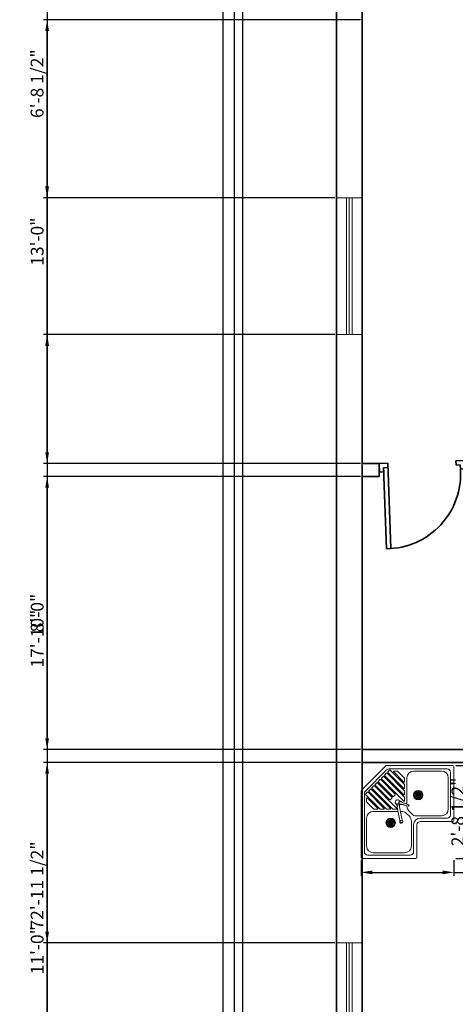
# Model space of a CAD drawing. Units: inches. Extents: x 1239 to 2276906, y 2273 to 321338.
# Tile 15 of 23: x 1239 to 1392, y 3026 to 3372. Entities that reach past the tile are written whole.
import ezdxf

# ---------------------------------------------------------------- set-up
doc = ezdxf.new("R2010")
doc.units = ezdxf.units.IN
for name, color, linetype, lineweight in [('A-ANNO-DIMS', 2, 'Continuous', 18), ('A-FLOR-FIXT', 9, 'Continuous', 18), ('C-PROP', 7, 'Continuous', 25), ('DOOR', 1, 'Continuous', 25), ('wall', 7, 'Continuous', 35), ('WINDOW', 50, 'Continuous', 18)]:
    doc.layers.add(name, color=color, linetype=linetype, lineweight=lineweight)
doc.styles.get("Standard").update_dxf_attribs({"font": 'arial.ttf'})
doc.dimstyles.new('ISO-25', dxfattribs={"dimtxt": 4.5, "dimasz": 4, "dimexe": 1.25, "dimexo": 0.625, "dimtad": 1, "dimdec": 1, "dimlunit": 3, "dimtxsty": 'Standard', "dimcen": 2.5, "dimadec": 0, "dimazin": 0, "dimtfac": 1, "dimtdec": 1, "dimtmove": 0, "dimatfit": 3, "dimfxl": 1, "dimarcsym": 0})

# ---------------------------------------------------------------- blocks, each defined once
blk = doc.blocks.new('new block')
for p, q in [((1.5, 1.5), (1.5, 30)), ((3, 0), (3, 30)), ((0, 3), (0, 0)), ((1.5, 3), (0, 3)), ((0, 0), (3, 0)), ((1.5, 1.5), (1.5, 3)), ((3, 1.5), (1.5, 1.5)), ((3, 0), (3, 1.5)), ((27, 0), (27, 1.5)), ((27, 1.5), (28.5, 1.5)), ((30, 0), (27, 0)), ((28.5, 1.5), (28.5, 3)), ((28.5, 3), (30, 3)), ((30, 3), (30, 0))]:
    blk.add_line(p, q)
blk.add_arc((2.25, 3.75), 26.26, 358.3634, 91.6366)
blk = doc.blocks.new('2.6door')
at = {"layer": 'wall'}
blk.add_blockref('new block', (0, 0), dxfattribs=at)
blk = doc.blocks.new('A$C4E531579')
for p, q in [((222.1, 827.1), (2.9, 607.9)), ((228.6, 791.2), (38.8, 601.4)), ((229.1, 830), (820, 830)), ((249.9, 800), (770, 800)), ((830, 820), (830, 340)), ((169.1, 703.4), (154.9, 689.2)), ((305.1, 574.4), (176.1, 703.4)), ((197.4, 731.6), (183.2, 717.5)), ((381.5, 512.2), (183.2, 710.4)), ((388.5, 547.5), (204.4, 731.6)), ((225.6, 759.9), (211.5, 745.8)), ((381.5, 568.7), (211.5, 738.7)), ((388.5, 604.1), (232.7, 759.9)), ((253.9, 788.2), (239.8, 774.1)), ((381.5, 625.3), (239.8, 767)), ((388.5, 660.7), (261, 788.2)), ((381.5, 681.9), (291.9, 771.5)), ((295.4, 780), (323.7, 780)), ((388.5, 717.2), (327.2, 778.5)), ((390, 713.7), (390, 685.4)), ((410, 720), (410, 483.9)), ((720, 780), (470, 780)), ((780, 440), (780, 720)), ((800, 770), (800, 390)), ((70.1, 604.4), (84.2, 618.5)), ((261.3, 448.5), (91.3, 618.5)), ((98.4, 632.6), (112.5, 646.8)), ((282.5, 441.5), (98.4, 625.6)), ((317.8, 448.5), (119.6, 646.8)), ((126.6, 660.9), (140.8, 675.1)), ((255.6, 524.9), (126.6, 653.9)), ((276.8, 546.1), (147.9, 675.1)), ((283.9, 553.2), (154.9, 682.1)), ((390, 657.1), (390, 628.8)), ((0, 10), (0, 600.9)), ((30, 60), (30, 580.1)), ((41.8, 576.1), (55.9, 590.2)), ((169.3, 441.5), (41.8, 569)), ((50, 534.6), (50, 506.3)), ((148.1, 448.5), (58.5, 538.1)), ((204.7, 448.5), (63, 590.2)), ((225.9, 441.5), (70.1, 597.3)), ((262.7, 524.9), (276.8, 539)), ((305.1, 567.3), (291, 553.2)), ((390, 600.6), (390, 572.3)), ((390, 544), (390, 515.7)), ((112.8, 441.5), (51.5, 502.8)), ((116.3, 440), (144.6, 440)), ((172.9, 440), (201.2, 440)), ((229.4, 440), (257.7, 440)), ((286, 440), (314.3, 440)), ((344.7, 353.4), (324.5, 455.5)), ((344.5, 460.1), (364.9, 357.1)), ((410, 468.8), (410, 466.1)), ((50, 110), (50, 360)), ((110, 420), (331.5, 420)), ((352.4, 420), (363.9, 420)), ((406.4, 402.4), (432.4, 376.4)), ((427.6, 423.6), (453.6, 397.6)), ((496.1, 380), (720, 380)), ((530, 360), (770, 360)), ((450, 333.9), (450, 110)), ((470, 300), (470, 60)), ((500, 300), (500, 10)), ((530, 330), (820, 330)), ((440, 30), (60, 30)), ((390, 50), (110, 50)), ((490, 0), (10, 0))]:
    blk.add_line(p, q)
for centre, radius in [((511.9, 565), 41.9), ((511.9, 565), 34.4), ((511.9, 565), 5.37), ((265, 318.1), 41.9), ((265, 318.1), 34.4), ((265, 318.1), 5.37)]:
    blk.add_circle(centre, radius)
for centre, radius, start, end in [((229.1, 820), 10, 90, 135), ((249.9, 770), 30, 90, 135), ((770, 770), 30, 0, 90), ((820, 820), 10, 0, 90), ((172.6, 699.8), 5, 45, 135), ((186.7, 714), 5, 135, 225), ((200.9, 728.1), 5, 45, 135), ((215, 742.2), 5, 135, 225), ((229.2, 756.4), 5, 45, 135), ((243.3, 770.5), 5, 135, 225), ((257.5, 784.7), 5, 45, 135), ((295.4, 775), 5, 90, 225), ((323.7, 775), 5, 45, 90), ((385, 713.7), 5, 0, 45), ((470, 720), 60, 90, 180), ((720, 720), 60, 0, 90), ((87.8, 615), 5, 45, 135), ((101.9, 629.1), 5, 135, 225), ((116, 643.3), 5, 45, 135), ((130.2, 657.4), 5, 135, 225), ((144.3, 671.5), 5, 45, 135), ((158.5, 685.7), 5, 135, 225), ((385, 685.4), 5, 225, 0), ((385, 628.8), 5, 225, 0), ((385, 657.1), 5, 0, 45), ((10, 600.9), 10, 135, 180), ((60, 580.1), 30, 135, 180), ((45.3, 572.5), 5, 135, 225), ((55, 534.6), 5, 45, 180), ((59.5, 586.7), 5, 45, 135), ((73.6, 600.8), 5, 135, 225), ((273.3, 542.6), 5, 315, 45), ((287.4, 556.7), 5, 225, 315), ((301.6, 570.8), 5, 315, 45), ((385, 572.3), 5, 225, 0), ((385, 600.6), 5, 0, 45), ((385, 544), 5, 0, 45), ((55, 506.3), 5, 180, 225), ((116.3, 445), 5, 225, 270), ((144.6, 445), 5, 270, 45), ((172.9, 445), 5, 225, 270), ((201.2, 445), 5, 270, 45), ((229.4, 445), 5, 225, 270), ((259.2, 528.4), 5, 225, 315), ((257.7, 445), 5, 270, 45), ((286, 445), 5, 225, 270), ((325.6, 504.4), 20, 52.72293, 268.78568), ((226.1, 437.3), 100, 10.4867, 33.97381), ((314.3, 445), 5, 270, 45), ((296.1, 462.7), 29.3, 9.84672, 38.35374), ((282.9, 16.5), 469.7, 72.94476, 84.83287), ((326.2, 504.9), 16.2, 278.92915, 32.15573), ((305.7, 211.8), 277.4, 72.23491, 84.23498), ((583, 916.9), 466.4, 238.27092, 250.20216), ((368.8, 476.8), 29.3, 168.25085, 191.99309), ((479.5, 750.1), 274.6, 239.9645, 252.02573), ((442.8, 478.3), 100, 177.65932, 190.48676), ((385, 515.7), 5, 225, 0), ((470, 466.1), 60, 180, 225), ((422.7, 471.9), 6.64, 252.6444, 68.86421), ((420.8, 471.6), 4.91, 314.25167, 37.23492), ((720, 440), 60, 270, 0), ((110, 360), 60, 90, 180), ((246.4, 335.2), 100, 355.98426, 10.4867), ((363.9, 360), 60, 45, 90), ((463.2, 375.3), 100, 190.48676, 204.98921), ((390, 333.9), 60, 0, 45), ((496.1, 440), 60, 225, 270), ((530, 300), 60, 90, 180), ((770, 390), 30, 270, 0), ((360, 327.2), 13.9, 175.98426, 24.98921), ((359.8, 327.5), 8.12, 180.36355, 342.44433), ((359, 332), 7.59, 72.42297, 131.67578), ((530, 300), 30, 90, 180), ((820, 340), 10, 270, 0), ((110, 110), 60, 180, 270), ((390, 110), 60, 270, 0), ((10, 10), 10, 180, 270), ((60, 60), 30, 180, 270), ((440, 60), 30, 270, 0), ((490, 10), 10, 270, 0)]:
    blk.add_arc(centre, radius, start, end)
at = {"extrusion": (0, -1e-16, -1)}
for centre, major_axis in [((492, 565), (14.5, 0)), ((511.9, 545.1), (0, 14.5))]:
    blk.add_ellipse(centre, major_axis=major_axis, ratio=0.137964, dxfattribs=at)
at = {"extrusion": (-1e-16, -2e-16, -1)}
blk.add_ellipse((494.7, 574.9), major_axis=(12.6, -7.2), ratio=0.137964, dxfattribs=at)
at = {"extrusion": (0, -2e-16, -1)}
for centre, major_axis in [((494.7, 555.1), (12.6, 7.2)), ((529.1, 574.9), (-12.6, -7.2))]:
    blk.add_ellipse(centre, major_axis=major_axis, ratio=0.137964, dxfattribs=at)
at = {"extrusion": (0, 0, -1)}
for centre, major_axis in [((501.9, 582.2), (7.2, -12.6)), ((511.9, 584.9), (0, -14.5)), ((521.8, 547.8), (-7.2, 12.6))]:
    blk.add_ellipse(centre, major_axis=major_axis, ratio=0.137964, dxfattribs=at)
at = {"extrusion": (-3e-16, 1e-16, -1)}
blk.add_ellipse((501.9, 547.8), major_axis=(7.2, 12.6), ratio=0.137964, dxfattribs=at)
at = {"extrusion": (3e-16, -1e-16, -1)}
blk.add_ellipse((521.8, 582.2), major_axis=(-7.2, -12.6), ratio=0.137964, dxfattribs=at)
at = {"extrusion": (-1e-16, -1e-16, -1)}
blk.add_ellipse((529.1, 555.1), major_axis=(-12.6, 7.2), ratio=0.137964, dxfattribs=at)
at = {"extrusion": (1e-16, -1e-16, -1)}
blk.add_ellipse((531.7, 565), major_axis=(-14.5, 0), ratio=0.137964, dxfattribs=at)
for centre, major_axis in [((265, 338), (0, -14.5)), ((245.1, 318.1), (14.5, 0)), ((247.8, 328.1), (12.6, -7.2)), ((247.8, 308.2), (12.6, 7.2)), ((255.1, 335.3), (7.2, -12.6)), ((255.1, 300.9), (7.2, 12.6)), ((265, 298.3), (0, 14.5)), ((274.9, 335.3), (-7.2, -12.6)), ((274.9, 300.9), (-7.2, 12.6)), ((282.2, 328.1), (-12.6, -7.2)), ((282.2, 308.2), (-12.6, 7.2)), ((284.9, 318.1), (-14.5, 0))]:
    blk.add_ellipse(centre, major_axis=major_axis, ratio=0.137964)
blk = doc.blocks.new('WIN-48')
for p, q in [((0, 48), (9, 48)), ((0, 0), (0, 48)), ((3.5, 0), (3.5, 48)), ((4.5, 0), (4.5, 48)), ((5.5, 0), (5.5, 48)), ((9, 0), (9, 48)), ((0, 0), (9, 0))]:
    blk.add_line(p, q)
blk = doc.blocks.new('*D66')
at = {"layer": 'A-ANNO-DIMS', "color": 0, "lineweight": -2, "transparency": 16777216}
for p, q in [((1358.99, 3077.03), (1358.99, 3071.51)), ((1391.67, 3077.03), (1391.67, 3071.51)), ((1362.99, 3072.76), (1387.67, 3072.76)), ((1391.67, 3072.76), (1435.76, 3072.76))]:
    blk.add_line(p, q, dxfattribs=at)
at = {"layer": 'A-ANNO-DIMS', "color": 0, "transparency": 16777216}
for points in [[(1362.99, 3073.42), (1362.99, 3072.09), (1358.99, 3072.76)], [(1387.67, 3073.42), (1387.67, 3072.09), (1391.67, 3072.76)]]:
    blk.add_solid(points, dxfattribs=at)
at = {"layer": 'Defpoints', "color": 0, "transparency": 16777216}
for p in [(1358.99, 3077.66), (1391.67, 3077.66), (1391.67, 3072.76)]:
    blk.add_point(p, dxfattribs=at)
at = {"layer": 'A-ANNO-DIMS', "color": 0, "transparency": 16777216, "insert": (1415.71, 3075.71), "char_height": 4.5, "attachment_point": 5}
blk.add_mtext('SINK 2\'-8 1/2"', dxfattribs=at)
blk = doc.blocks.new('*D67')
at = {"layer": 'A-ANNO-DIMS', "color": 0, "lineweight": -2, "transparency": 16777216}
for p, q in [((1392.29, 3110.33), (1397.82, 3110.33)), ((1396.57, 3081.66), (1396.57, 3106.33)), ((1392.29, 3077.66), (1397.82, 3077.66))]:
    blk.add_line(p, q, dxfattribs=at)
at = {"layer": 'A-ANNO-DIMS', "color": 0, "transparency": 16777216}
for points in [[(1395.9, 3106.33), (1397.24, 3106.33), (1396.57, 3110.33)], [(1395.9, 3081.66), (1397.24, 3081.66), (1396.57, 3077.66)]]:
    blk.add_solid(points, dxfattribs=at)
at = {"layer": 'Defpoints', "color": 0, "transparency": 16777216}
for p in [(1391.67, 3110.33), (1396.57, 3110.33), (1391.67, 3077.66)]:
    blk.add_point(p, dxfattribs=at)
at = {"layer": 'A-ANNO-DIMS', "color": 0, "transparency": 16777216, "insert": (1393.62, 3094), "char_height": 4.5, "attachment_point": 5, "rotation": 90}
blk.add_mtext('2\'-8 1/2"', dxfattribs=at)
blk = doc.blocks.new('*D82')
at = {"layer": 'A-ANNO-DIMS', "color": 0, "lineweight": -2, "transparency": 16777216}
for p, q in [((1349.76, 3505.9), (1247.33, 3505.9)), ((1248.58, 3501.9), (1248.58, 2634.4)), ((1358.76, 2630.4), (1247.33, 2630.4))]:
    blk.add_line(p, q, dxfattribs=at)
at = {"layer": 'A-ANNO-DIMS', "color": 0, "transparency": 16777216}
for points in [[(1247.92, 3501.9), (1249.25, 3501.9), (1248.58, 3505.9)], [(1247.92, 2634.4), (1249.25, 2634.4), (1248.58, 2630.4)]]:
    blk.add_solid(points, dxfattribs=at)
at = {"layer": 'Defpoints', "color": 0, "transparency": 16777216}
for p in [(1350.38, 3505.9), (1248.58, 2630.4), (1359.38, 2630.4)]:
    blk.add_point(p, dxfattribs=at)
at = {"layer": 'A-ANNO-DIMS', "color": 0, "transparency": 16777216, "insert": (1245.63, 3068.15), "char_height": 4.5, "attachment_point": 5, "rotation": 90}
blk.add_mtext('72\'-11 1/2"', dxfattribs=at)
blk = doc.blocks.new('*D89')
at = {"layer": 'A-ANNO-DIMS', "color": 0, "lineweight": -2, "transparency": 16777216}
for p, q in [((1359.38, 3215.77), (1359.38, 2275.7)), ((1551.38, 3215.77), (1551.38, 2275.7)), ((1363.38, 2276.95), (1547.38, 2276.95))]:
    blk.add_line(p, q, dxfattribs=at)
at = {"layer": 'A-ANNO-DIMS', "color": 0, "transparency": 16777216}
for points in [[(1363.38, 2277.61), (1363.38, 2276.28), (1359.38, 2276.95)], [(1547.38, 2277.61), (1547.38, 2276.28), (1551.38, 2276.95)]]:
    blk.add_solid(points, dxfattribs=at)
at = {"layer": 'Defpoints', "color": 0, "transparency": 16777216}
for p in [(1359.38, 3216.4), (1551.38, 3216.4), (1551.38, 2276.95)]:
    blk.add_point(p, dxfattribs=at)
at = {"layer": 'A-ANNO-DIMS', "color": 0, "transparency": 16777216, "insert": (1455.38, 2279.87), "char_height": 4.5, "attachment_point": 5}
blk.add_mtext('16\'-0"', dxfattribs=at)
blk = doc.blocks.new('*D90')
at = {"layer": 'A-ANNO-DIMS', "color": 0, "lineweight": -2, "transparency": 16777216}
for p, q in [((1358.76, 3372.4), (1247.33, 3372.4)), ((1248.58, 3220.4), (1248.58, 3368.4)), ((1358.76, 3216.4), (1247.33, 3216.4))]:
    blk.add_line(p, q, dxfattribs=at)
at = {"layer": 'A-ANNO-DIMS', "color": 0, "transparency": 16777216}
for points in [[(1247.92, 3368.4), (1249.25, 3368.4), (1248.58, 3372.4)], [(1247.92, 3220.4), (1249.25, 3220.4), (1248.58, 3216.4)]]:
    blk.add_solid(points, dxfattribs=at)
at = {"layer": 'Defpoints', "color": 0, "transparency": 16777216}
for p in [(1248.58, 3372.4), (1359.38, 3372.4), (1359.38, 3216.4)]:
    blk.add_point(p, dxfattribs=at)
at = {"layer": 'A-ANNO-DIMS', "color": 0, "transparency": 16777216, "insert": (1245.66, 3294.4), "char_height": 4.5, "attachment_point": 5, "rotation": 90}
blk.add_mtext('13\'-0"', dxfattribs=at)
blk = doc.blocks.new('*D91')
at = {"layer": 'A-ANNO-DIMS', "color": 0, "lineweight": -2, "transparency": 16777216}
for p, q in [((1359.38, 3116.52), (1359.38, 3608.95)), ((1451.38, 3106.02), (1451.38, 3608.95)), ((1363.38, 3607.7), (1447.38, 3607.7))]:
    blk.add_line(p, q, dxfattribs=at)
at = {"layer": 'A-ANNO-DIMS', "color": 0, "transparency": 16777216}
for points in [[(1363.38, 3608.36), (1363.38, 3607.03), (1359.38, 3607.7)], [(1447.38, 3608.36), (1447.38, 3607.03), (1451.38, 3607.7)]]:
    blk.add_solid(points, dxfattribs=at)
at = {"layer": 'Defpoints', "color": 0, "transparency": 16777216}
for p in [(1451.38, 3607.7), (1359.38, 3115.9), (1451.38, 3105.4)]:
    blk.add_point(p, dxfattribs=at)
at = {"layer": 'A-ANNO-DIMS', "color": 0, "transparency": 16777216, "insert": (1405.38, 3610.62), "char_height": 4.5, "attachment_point": 5}
blk.add_mtext('7\'-8"', dxfattribs=at)
blk = doc.blocks.new('*D92')
at = {"layer": 'A-ANNO-DIMS', "color": 0, "lineweight": -2, "transparency": 16777216}
for p, q in [((1358.76, 3211.9), (1247.33, 3211.9)), ((1248.58, 3119.9), (1248.58, 3207.9)), ((1358.76, 3115.9), (1247.33, 3115.9))]:
    blk.add_line(p, q, dxfattribs=at)
at = {"layer": 'A-ANNO-DIMS', "color": 0, "transparency": 16777216}
for points in [[(1247.92, 3207.9), (1249.25, 3207.9), (1248.58, 3211.9)], [(1247.92, 3119.9), (1249.25, 3119.9), (1248.58, 3115.9)]]:
    blk.add_solid(points, dxfattribs=at)
at = {"layer": 'Defpoints', "color": 0, "transparency": 16777216}
for p in [(1248.58, 3211.9), (1359.38, 3211.9), (1359.38, 3115.9)]:
    blk.add_point(p, dxfattribs=at)
at = {"layer": 'A-ANNO-DIMS', "color": 0, "transparency": 16777216, "insert": (1245.66, 3163.9), "char_height": 4.5, "attachment_point": 5, "rotation": 90}
blk.add_mtext('8\'-0"', dxfattribs=at)
blk = doc.blocks.new('*D93')
at = {"layer": 'A-ANNO-DIMS', "color": 0, "lineweight": -2, "transparency": 16777216}
for p, q in [((1358.76, 3111.4), (1247.33, 3111.4)), ((1248.58, 2983.4), (1248.58, 3107.4)), ((1358.76, 2979.4), (1247.33, 2979.4))]:
    blk.add_line(p, q, dxfattribs=at)
at = {"layer": 'A-ANNO-DIMS', "color": 0, "transparency": 16777216}
for points in [[(1247.92, 3107.4), (1249.25, 3107.4), (1248.58, 3111.4)], [(1247.92, 2983.4), (1249.25, 2983.4), (1248.58, 2979.4)]]:
    blk.add_solid(points, dxfattribs=at)
at = {"layer": 'Defpoints', "color": 0, "transparency": 16777216}
for p in [(1248.58, 3111.4), (1359.38, 3111.4), (1359.38, 2979.4)]:
    blk.add_point(p, dxfattribs=at)
at = {"layer": 'A-ANNO-DIMS', "color": 0, "transparency": 16777216, "insert": (1245.66, 3045.4), "char_height": 4.5, "attachment_point": 5, "rotation": 90}
blk.add_mtext('11\'-0"', dxfattribs=at)
blk = doc.blocks.new('*D102')
at = {"layer": 'A-ANNO-DIMS', "color": 0, "lineweight": -2, "transparency": 16777216}
for p, q in [((1317.38, 2608.14), (1317.38, 3608.95)), ((1540.55, 2608.14), (1540.55, 3608.95)), ((1321.38, 3607.7), (1536.55, 3607.7))]:
    blk.add_line(p, q, dxfattribs=at)
at = {"layer": 'A-ANNO-DIMS', "color": 0, "transparency": 16777216}
for points in [[(1321.38, 3608.36), (1321.38, 3607.03), (1317.38, 3607.7)], [(1536.55, 3608.36), (1536.55, 3607.03), (1540.55, 3607.7)]]:
    blk.add_solid(points, dxfattribs=at)
at = {"layer": 'Defpoints', "color": 0, "transparency": 16777216}
for p in [(1540.55, 3607.7), (1317.38, 2607.52), (1540.55, 2607.52)]:
    blk.add_point(p, dxfattribs=at)
at = {"layer": 'A-ANNO-DIMS', "color": 0, "transparency": 16777216, "insert": (1428.97, 3610.62), "char_height": 4.5, "attachment_point": 5}
blk.add_mtext('18\'-7"', dxfattribs=at)
blk = doc.blocks.new('*D105')
at = {"layer": 'A-ANNO-DIMS', "color": 0, "lineweight": -2, "transparency": 16777216}
for p, q in [((1349.76, 3390.05), (1247.33, 3390.05)), ((1248.58, 3386.05), (1248.58, 3313.78)), ((1349.76, 3309.78), (1247.33, 3309.78))]:
    blk.add_line(p, q, dxfattribs=at)
at = {"layer": 'A-ANNO-DIMS', "color": 0, "transparency": 16777216}
for points in [[(1247.92, 3386.05), (1249.25, 3386.05), (1248.58, 3390.05)], [(1247.92, 3313.78), (1249.25, 3313.78), (1248.58, 3309.78)]]:
    blk.add_solid(points, dxfattribs=at)
at = {"layer": 'Defpoints', "color": 0, "transparency": 16777216}
for p in [(1350.38, 3390.05), (1248.58, 3309.78), (1350.38, 3309.78)]:
    blk.add_point(p, dxfattribs=at)
at = {"layer": 'A-ANNO-DIMS', "color": 0, "transparency": 16777216, "insert": (1245.63, 3349.91), "char_height": 4.5, "attachment_point": 5, "rotation": 90}
blk.add_mtext('6\'-8 1/2"', dxfattribs=at)
blk = doc.blocks.new('*D106')
at = {"layer": 'A-ANNO-DIMS', "color": 0, "lineweight": -2, "transparency": 16777216}
for p, q in [((1349.76, 3261.78), (1247.33, 3261.78)), ((1248.58, 3257.78), (1248.58, 3051.98)), ((1349.76, 3047.98), (1247.33, 3047.98))]:
    blk.add_line(p, q, dxfattribs=at)
at = {"layer": 'A-ANNO-DIMS', "color": 0, "transparency": 16777216}
for points in [[(1247.92, 3257.78), (1249.25, 3257.78), (1248.58, 3261.78)], [(1247.92, 3051.98), (1249.25, 3051.98), (1248.58, 3047.98)]]:
    blk.add_solid(points, dxfattribs=at)
at = {"layer": 'Defpoints', "color": 0, "transparency": 16777216}
for p in [(1350.38, 3261.78), (1248.58, 3047.98), (1350.38, 3047.98)]:
    blk.add_point(p, dxfattribs=at)
at = {"layer": 'A-ANNO-DIMS', "color": 0, "transparency": 16777216, "insert": (1245.66, 3154.88), "char_height": 4.5, "attachment_point": 5, "rotation": 90}
blk.add_mtext('17\'-10"', dxfattribs=at)

msp = doc.modelspace()

# ---------------------------------------------------------------- linework, layer by layer
at = {"layer": 'C-PROP'}
for points in [[(1970.38, 2345.9), (1970.38, 3545.9), (1310.38, 3545.9), (1310.38, 2345.9), (1644.79, 2345.9)], [(1966.38, 2349.9), (1966.38, 3541.9), (1314.38, 3541.9), (1314.38, 2607.52)]]:
    msp.add_lwpolyline(points, dxfattribs=at)
at = {"layer": 'wall'}
for p, q in [((1350.38, 3505.9), (1350.38, 2607.52)), ((1359.38, 3496.9), (1359.38, 3216.4)), ((1365.38, 3216.4), (1359.38, 3216.4)), ((1365.38, 3216.4), (1365.38, 3211.9)), ((1359.38, 3211.9), (1359.38, 2607.52)), ((1365.38, 3211.9), (1359.38, 3211.9)), ((1551.38, 3115.9), (1359.38, 3115.9)), ((1551.38, 3111.4), (1359.38, 3111.4))]:
    msp.add_line(p, q, dxfattribs=at)

# ---------------------------------------------------------------- block references
at = {"layer": 'A-FLOR-FIXT', "xscale": 0.0393700787401575, "yscale": 0.0393700787401575, "zscale": 0.0393700787401575}
msp.add_blockref('A$C4E531579', (1358.99, 3077.66), dxfattribs=at)
at = {"layer": 'DOOR', "xscale": -1, "rotation": 182.1398655045003}
msp.add_blockref('2.6door', (1365.38, 3216.4), dxfattribs=at)
at = {"layer": 'WINDOW'}
for p in [(1350.38, 3261.78), (1350.38, 2999.98)]:
    msp.add_blockref('WIN-48', p, dxfattribs=at)

# ---------------------------------------------------------------- dimensions: what is measured, and where the dimension line sits
at = {"layer": 'A-ANNO-DIMS'}
for base, p1, p2, picture, middle in [((1540.55, 3607.7), (1317.38, 2607.52), (1540.55, 2607.52), '*D102', (1428.97, 3610.62)), ((1451.38, 3607.7), (1359.38, 3115.9), (1451.38, 3105.4), '*D91', (1405.38, 3610.62)), ((1551.38, 2276.95), (1359.38, 3216.4), (1551.38, 3216.4), '*D89', (1455.38, 2279.87))]:
    dim = msp.add_linear_dim(base=base, p1=p1, p2=p2, dimstyle='ISO-25', override={"dimdec": 1, "dimlfac": 1, "dimrnd": 0, "dimzin": 1, "dimdsep": 46, "dimlunit": 4, "dimfrac": 2}, dxfattribs=at)
    dim.commit()
    dim.dimension.update_dxf_attribs({"geometry": picture, "text_midpoint": middle})
for base, p1, p2, picture, middle in [((1248.58, 2630.4), (1350.38, 3505.9), (1359.38, 2630.4), '*D82', (1245.63, 3068.15)), ((1248.58, 3309.78), (1350.38, 3390.05), (1350.38, 3309.78), '*D105', (1245.63, 3349.91)), ((1248.58, 3372.4), (1359.38, 3216.4), (1359.38, 3372.4), '*D90', (1245.66, 3294.4)), ((1248.58, 3047.98), (1350.38, 3261.78), (1350.38, 3047.98), '*D106', (1245.66, 3154.88)), ((1248.58, 3211.9), (1359.38, 3115.9), (1359.38, 3211.9), '*D92', (1245.66, 3163.9)), ((1248.58, 3111.4), (1359.38, 2979.4), (1359.38, 3111.4), '*D93', (1245.66, 3045.4)), ((1396.57, 3110.33), (1391.67, 3077.66), (1391.67, 3110.33), '*D67', (1393.62, 3094))]:
    dim = msp.add_linear_dim(base=base, p1=p1, p2=p2, angle=90, dimstyle='ISO-25', override={"dimdec": 1, "dimlfac": 1, "dimrnd": 0, "dimzin": 1, "dimdsep": 46, "dimlunit": 4, "dimfrac": 2}, dxfattribs=at)
    dim.commit()
    dim.dimension.update_dxf_attribs({"geometry": picture, "text_midpoint": middle})
dim = msp.add_linear_dim(base=(1391.67, 3072.76), p1=(1358.99, 3077.66), p2=(1391.67, 3077.66), text='SINK <>', dimstyle='ISO-25', override={"dimdec": 1, "dimlfac": 1, "dimrnd": 0, "dimzin": 1, "dimdsep": 46, "dimlunit": 4, "dimfrac": 2}, dxfattribs=at)
dim.commit()
dim.dimension.update_dxf_attribs({"geometry": '*D66', "text_midpoint": (1415.71, 3075.71)})

doc.saveas('drawing.dxf')
